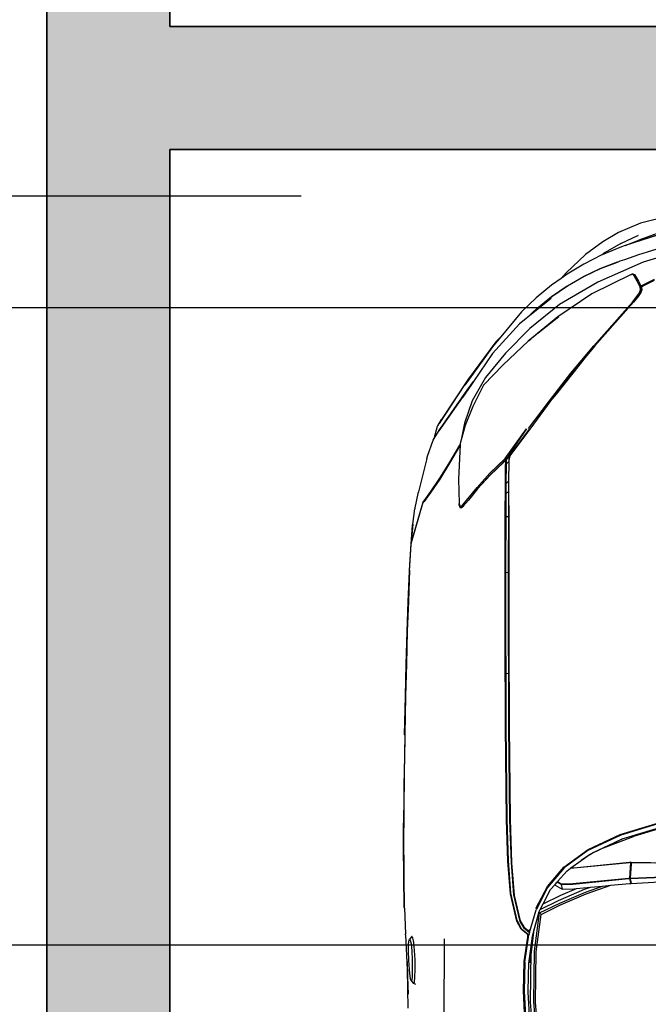
# Model space of a CAD drawing. Units: inches. Extents: x -4737294 to -4736756, y 1716389 to 1717040.
# Tile 12 of 25: x -4737217 to -4737171, y 1716597 to 1716669. Entities that reach past the tile are written whole.
import ezdxf

# ---------------------------------------------------------------- set-up
doc = ezdxf.new("R2010")
doc.units = ezdxf.units.IN
doc.header["$MEASUREMENT"] = 0
for name, color, linetype, lineweight in [('A-ANNO-DIMS', 2, 'Continuous', 18), ('A-EQPM-VEHI', 250, 'Continuous', 13), ('A-WALL-PATT', 244, 'Continuous', 13), ('walls', 252, 'Continuous', 35)]:
    doc.layers.add(name, color=color, linetype=linetype, lineweight=lineweight)
doc.layers.add('Edges', color=250, linetype='Continuous')
doc.styles.get("Standard").update_dxf_attribs({"font": 'arial.ttf'})
doc.dimstyles.get("Standard").update_dxf_attribs({"dimtxt": 8, "dimasz": 0.18, "dimexe": 0.18, "dimexo": 0.0625, "dimgap": 0.09, "dimtad": 0, "dimtih": 1, "dimtoh": 1, "dimzin": 0, "dimdsep": 46, "dimlunit": 3, "dimtxsty": 'Standard', "dimcen": 0.09, "dimadec": 0, "dimazin": 0, "dimtfac": 1, "dimtofl": 0, "dimtmove": 0, "dimatfit": 3, "dimfxl": 1, "dimtolj": 1, "dimtzin": 0, "dimarcsym": 0})

# ---------------------------------------------------------------- blocks, each defined once
blk = doc.blocks.new('Nissan Qashqai pl')
at = {"layer": 'Edges'}
for p, q in [((8.4086, 11.6764), (8.4045, 11.4011)), ((8.4305, 11.3996), (8.419, 11.6758)), ((8.4204, 11.6758), (8.4319, 11.3996)), ((8.4394, 11.4014), (8.4238, 11.6766)), ((7.3676, 11.5172), (7.3963, 11.4215)), ((8.3573, 11.3824), (8.3296, 11.4739)), ((8.3311, 11.4733), (8.3582, 11.3836)), ((8.3648, 11.3863), (8.3377, 11.4753)), ((8.3392, 11.4758), (8.3608, 11.4048)), ((7.3193, 11.4645), (7.3309, 11.4166)), ((7.344, 11.4572), (7.3596, 11.4139)), ((7.3467, 11.4596), (7.3686, 11.3913)), ((7.3489, 11.4517), (7.3686, 11.3913)), ((7.375, 11.4442), (7.3799, 11.4278)), ((7.4255, 11.4398), (7.4367, 11.4174)), ((7.4379, 11.4179), (7.4267, 11.4401)), ((8.4041, 11.4013), (8.4048, 11.4423)), ((7.3799, 11.4278), (7.3845, 11.4136)), ((7.3963, 11.4215), (7.4302, 11.3449)), ((7.3309, 11.4166), (7.347, 11.3798)), ((7.3655, 11.3837), (7.3514, 11.4133)), ((7.3686, 11.3913), (7.3596, 11.4139)), ((7.3845, 11.4136), (7.3925, 11.3899)), ((7.4167, 11.4049), (7.417, 11.4065)), ((7.4172, 11.4047), (7.4167, 11.4049)), ((7.4169, 11.4036), (7.4167, 11.4049)), ((7.4282, 11.4113), (7.4169, 11.4044)), ((7.417, 11.4065), (7.4283, 11.4135)), ((7.4183, 11.406), (7.4172, 11.4047)), ((7.4296, 11.4129), (7.4183, 11.406)), ((7.4387, 11.4162), (7.4282, 11.4113)), ((7.4283, 11.4135), (7.4359, 11.417)), ((7.4296, 11.4129), (7.4383, 11.417)), ((7.4359, 11.417), (7.4367, 11.4174)), ((7.4383, 11.417), (7.4367, 11.4174)), ((7.4375, 11.42), (7.4384, 11.4182)), ((7.4379, 11.4179), (7.4384, 11.4182)), ((7.4389, 11.4173), (7.4379, 11.4179)), ((7.4383, 11.417), (7.4379, 11.4179)), ((7.4389, 11.4173), (7.4383, 11.417)), ((7.4384, 11.4182), (7.4387, 11.4183)), ((7.4387, 11.4183), (7.443, 11.4188)), ((7.4431, 11.4166), (7.4387, 11.4162)), ((7.4389, 11.4173), (7.44, 11.4178)), ((7.4442, 11.4183), (7.44, 11.4178)), ((7.443, 11.4188), (7.4477, 11.4172)), ((7.4479, 11.4149), (7.4431, 11.4166)), ((7.4477, 11.4172), (7.4442, 11.4183)), ((7.4477, 11.4172), (7.4541, 11.4128)), ((7.4541, 11.4108), (7.4479, 11.4149)), ((7.4541, 11.4128), (7.4638, 11.4051)), ((7.4635, 11.4034), (7.4541, 11.4108)), ((7.4638, 11.4051), (7.5371, 11.34)), ((8.3799, 11.3545), (8.3608, 11.4048)), ((7.3686, 11.3913), (7.3707, 11.3849)), ((7.3925, 11.3899), (7.3938, 11.3859)), ((7.4172, 11.4047), (7.4169, 11.4044)), ((7.4169, 11.4044), (7.4169, 11.4036)), ((7.4172, 11.4018), (7.4169, 11.4036)), ((7.4169, 11.4036), (7.4169, 11.403)), ((7.4169, 11.403), (7.4172, 11.4011)), ((7.4174, 11.4013), (7.4172, 11.4018)), ((7.4172, 11.4011), (7.4498, 11.3349)), ((7.4174, 11.4013), (7.4175, 11.4012)), ((7.5369, 11.3385), (7.4635, 11.4034)), ((8.407, 11.401), (8.4037, 11.4002)), ((8.4037, 11.4002), (8.4314, 11.3985)), ((8.4037, 11.3992), (8.4037, 11.4002)), ((8.4037, 11.3992), (8.4046, 11.3981)), ((8.4042, 11.3983), (8.4037, 11.3992)), ((8.4041, 11.4013), (8.4045, 11.4011)), ((8.4134, 11.3049), (8.4042, 11.3983)), ((8.4045, 11.4011), (8.407, 11.401)), ((8.4046, 11.3981), (8.4138, 11.3048)), ((8.407, 11.401), (8.4305, 11.3996)), ((8.4305, 11.3996), (8.4319, 11.3996)), ((8.4306, 11.3966), (8.4314, 11.3975)), ((8.4398, 11.3032), (8.4306, 11.3966)), ((8.4314, 11.3985), (8.4394, 11.4004)), ((8.4314, 11.3985), (8.4314, 11.3975)), ((8.4314, 11.3975), (8.4319, 11.3967)), ((8.4319, 11.3996), (8.436, 11.4006)), ((8.4319, 11.3967), (8.4412, 11.3033)), ((8.436, 11.4006), (8.4394, 11.4014)), ((8.4394, 11.4004), (8.436, 11.4006)), ((8.4394, 11.3984), (8.4394, 11.4004)), ((8.4425, 11.3672), (8.4394, 11.3984)), ((7.347, 11.3798), (7.3624, 11.3535)), ((7.3655, 11.3837), (7.3805, 11.3576)), ((7.3707, 11.3849), (7.3843, 11.3522)), ((7.3938, 11.3859), (7.3951, 11.3822)), ((7.3951, 11.3822), (7.3965, 11.3787)), ((7.3962, 11.3781), (7.3965, 11.3787)), ((7.4071, 11.3493), (7.3962, 11.3781)), ((7.3965, 11.3787), (7.3969, 11.3777)), ((7.3969, 11.3777), (7.4078, 11.349)), ((8.3826, 11.3291), (8.3573, 11.3824)), ((8.3582, 11.3836), (8.3844, 11.3284)), ((8.3646, 11.387), (8.3799, 11.3545)), ((8.3888, 11.3355), (8.3648, 11.3863)), ((7.3805, 11.3576), (7.3843, 11.3522)), ((8.4571, 11.3258), (8.4425, 11.3672)), ((8.4439, 11.3531), (8.4425, 11.3672)), ((7.3624, 11.3535), (7.3837, 11.3245)), ((7.3843, 11.3522), (7.3845, 11.3517)), ((7.3845, 11.3517), (7.3997, 11.3215)), ((7.4205, 11.3212), (7.4071, 11.3493)), ((7.4078, 11.349), (7.4211, 11.321)), ((7.4302, 11.3449), (7.4679, 11.2807)), ((7.5371, 11.34), (7.5568, 11.324)), ((8.3799, 11.3545), (8.3888, 11.3355)), ((8.454, 11.3245), (8.4439, 11.3531)), ((8.4459, 11.3326), (8.4439, 11.3531)), ((7.3837, 11.3245), (7.4147, 11.2918)), ((7.4498, 11.3349), (7.4884, 11.2778)), ((7.5827, 11.3001), (7.5369, 11.3385)), ((7.584, 11.3013), (7.5568, 11.324)), ((7.5568, 11.324), (7.5829, 11.303)), ((8.4122, 11.2883), (8.3826, 11.3291)), ((8.3844, 11.3284), (8.4134, 11.2888)), ((8.3901, 11.3328), (8.3888, 11.3355)), ((8.3901, 11.3328), (8.4011, 11.3173)), ((8.3904, 11.3321), (8.3901, 11.3328)), ((8.4011, 11.3173), (8.3904, 11.3321)), ((8.4493, 11.3229), (8.4459, 11.3326)), ((8.4482, 11.3095), (8.4459, 11.3326)), ((8.468, 11.2793), (8.4493, 11.3229)), ((8.4725, 11.2812), (8.454, 11.3245)), ((8.4756, 11.2826), (8.4571, 11.3258)), ((7.3997, 11.3215), (7.4166, 11.2939)), ((7.4363, 11.294), (7.4205, 11.3212)), ((7.4211, 11.321), (7.4369, 11.2938)), ((8.4135, 11.3), (8.4011, 11.3173)), ((8.4594, 11.2831), (8.4482, 11.3095)), ((8.4487, 11.305), (8.4482, 11.3095)), ((7.4147, 11.2918), (7.4239, 11.2837)), ((7.4166, 11.2939), (7.4239, 11.2837)), ((7.4542, 11.2677), (7.4363, 11.294)), ((7.4369, 11.2938), (7.4549, 11.2675)), ((7.6296, 11.2639), (7.5827, 11.3001)), ((7.5829, 11.303), (7.618, 11.275)), ((7.618, 11.275), (7.584, 11.3013)), ((8.4135, 11.3), (8.4134, 11.3049)), ((8.4139, 11.2994), (8.4135, 11.3)), ((8.4138, 11.3048), (8.4139, 11.2994)), ((8.4183, 11.2934), (8.4139, 11.2994)), ((8.4365, 11.2776), (8.4183, 11.2934)), ((8.44, 11.2834), (8.4398, 11.3032)), ((8.4412, 11.3033), (8.4415, 11.2835)), ((8.4489, 11.2852), (8.4487, 11.305)), ((7.4239, 11.2837), (7.4354, 11.2675)), ((7.4679, 11.2807), (7.5081, 11.2311)), ((7.4882, 11.2797), (7.5243, 11.2341)), ((7.4884, 11.2778), (7.5289, 11.2283)), ((7.618, 11.275), (7.6301, 11.2654)), ((8.4444, 11.2608), (8.4122, 11.2883)), ((8.4134, 11.2888), (8.4462, 11.2609)), ((8.4365, 11.2776), (8.44, 11.2834)), ((8.4375, 11.2767), (8.4365, 11.2776)), ((8.4415, 11.2835), (8.4375, 11.2767)), ((8.4412, 11.2735), (8.4375, 11.2767)), ((8.4422, 11.2737), (8.4412, 11.2735)), ((8.4499, 11.2659), (8.4412, 11.2735)), ((8.4415, 11.2835), (8.4489, 11.2852)), ((8.4422, 11.2737), (8.4489, 11.2852)), ((8.4737, 11.2534), (8.4594, 11.2831)), ((8.4831, 11.2484), (8.468, 11.2793)), ((8.4889, 11.2473), (8.4725, 11.2812)), ((8.4914, 11.25), (8.4756, 11.2826)), ((7.4354, 11.2675), (7.4565, 11.2419)), ((7.4744, 11.2427), (7.4542, 11.2677)), ((7.4549, 11.2675), (7.475, 11.2426)), ((7.4574, 11.267), (7.4885, 11.2283)), ((7.676, 11.2289), (7.6296, 11.2639)), ((7.6301, 11.2654), (7.6306, 11.2651)), ((7.6306, 11.2651), (7.6306, 11.265)), ((7.6306, 11.265), (7.6373, 11.2601)), ((7.6373, 11.2601), (7.6769, 11.2312)), ((8.4814, 11.2413), (8.4444, 11.2608)), ((8.4462, 11.2609), (8.4838, 11.2415)), ((8.4737, 11.2534), (8.4499, 11.2659)), ((7.4565, 11.2419), (7.4801, 11.2168)), ((7.4918, 11.2242), (7.4744, 11.2427)), ((7.475, 11.2426), (7.477, 11.2404)), ((7.477, 11.2404), (7.4765, 11.2411)), ((7.477, 11.2405), (7.4775, 11.2399)), ((7.4784, 11.2388), (7.477, 11.2404)), ((7.477, 11.2404), (7.4775, 11.2399)), ((7.4775, 11.2399), (7.4787, 11.2385)), ((7.4775, 11.2399), (7.4787, 11.2387)), ((8.4831, 11.2484), (8.4737, 11.2534)), ((8.4867, 11.2465), (8.4831, 11.2484)), ((8.5216, 11.2303), (8.4838, 11.2415)), ((8.528, 11.2354), (8.4867, 11.2465)), ((8.5214, 11.2374), (8.4867, 11.2465)), ((8.4889, 11.2473), (8.4914, 11.25)), ((8.5531, 11.2387), (8.4889, 11.2473)), ((8.5544, 11.2416), (8.4914, 11.25)), ((8.6386, 11.2404), (8.5544, 11.2416)), ((8.7481, 11.2473), (8.6375, 11.2376)), ((8.7491, 11.2501), (8.6386, 11.2404)), ((7.4787, 11.2387), (7.4782, 11.2392)), ((7.4795, 11.2377), (7.4787, 11.2387)), ((7.4787, 11.2387), (7.4885, 11.2283)), ((7.4885, 11.2283), (7.4918, 11.2242)), ((7.4918, 11.2242), (7.5001, 11.2139)), ((7.5081, 11.2311), (7.5492, 11.1902)), ((7.5243, 11.2341), (7.5286, 11.2296)), ((7.5289, 11.2283), (7.5687, 11.1862)), ((7.7261, 11.1898), (7.6762, 11.2256)), ((7.6762, 11.2256), (7.7233, 11.1928)), ((7.6769, 11.2312), (7.7194, 11.1992)), ((7.7232, 11.1955), (7.6771, 11.2307)), ((8.5125, 11.221), (8.5177, 11.2272)), ((8.5132, 11.2202), (8.5216, 11.2303)), ((8.5155, 11.2168), (8.5258, 11.2291)), ((8.5237, 11.2252), (8.5163, 11.2162)), ((8.5197, 11.2297), (8.5166, 11.2307)), ((8.5177, 11.2272), (8.5197, 11.2297)), ((8.5216, 11.2303), (8.5197, 11.2297)), ((8.5214, 11.2374), (8.555, 11.233)), ((8.5301, 11.2352), (8.5214, 11.2374)), ((8.5216, 11.2303), (8.5258, 11.2291)), ((8.5259, 11.2279), (8.5237, 11.2252)), ((8.5258, 11.2291), (8.5259, 11.2279)), ((8.5715, 11.2227), (8.5258, 11.2291)), ((8.5294, 11.2274), (8.5259, 11.2279)), ((8.5736, 11.2291), (8.528, 11.2354)), ((8.5706, 11.2216), (8.5294, 11.2274)), ((8.6375, 11.2376), (8.5531, 11.2387)), ((8.6387, 11.2319), (8.555, 11.233)), ((8.555, 11.233), (8.5726, 11.2307)), ((8.5941, 11.2286), (8.5736, 11.2291)), ((8.5941, 11.2289), (8.5941, 11.2286)), ((8.622, 11.228), (8.5941, 11.2286)), ((8.6203, 11.2213), (8.6721, 11.2241)), ((8.6699, 11.231), (8.622, 11.228)), ((8.6721, 11.2348), (8.6387, 11.2319)), ((7.4801, 11.2168), (7.5217, 11.1823)), ((7.5001, 11.2139), (7.5501, 11.1684)), ((8.5018, 11.2098), (8.4559, 11.1991)), ((8.5029, 11.2092), (8.4571, 11.1983)), ((8.4588, 11.2036), (8.5032, 11.2141)), ((8.4595, 11.2047), (8.5025, 11.2148)), ((8.5155, 11.2168), (8.5018, 11.2098)), ((8.5025, 11.2148), (8.5125, 11.221)), ((8.5163, 11.2162), (8.5029, 11.2092)), ((8.5032, 11.2141), (8.5132, 11.2202)), ((8.6197, 11.2201), (8.5706, 11.2216)), ((8.5715, 11.2227), (8.6203, 11.2213)), ((8.6683, 11.2226), (8.6197, 11.2201)), ((7.5492, 11.1902), (7.59, 11.1565)), ((7.7194, 11.1992), (7.7232, 11.1966)), ((7.7232, 11.1966), (7.7279, 11.1965)), ((7.7281, 11.1918), (7.7232, 11.1955)), ((7.7232, 11.1955), (7.7245, 11.1955)), ((7.7267, 11.1902), (7.7233, 11.1928)), ((7.7247, 11.1954), (7.7245, 11.1955)), ((7.7245, 11.1955), (7.7294, 11.1955)), ((7.7286, 11.1881), (7.7267, 11.1902)), ((7.7281, 11.1918), (7.7299, 11.1904)), ((7.7349, 11.1917), (7.7281, 11.1918)), ((7.753, 11.1648), (7.7281, 11.1918)), ((7.7294, 11.1955), (7.731, 11.1955)), ((7.7299, 11.1904), (7.7324, 11.1876)), ((7.7299, 11.1904), (7.7364, 11.1904)), ((7.731, 11.1955), (7.7349, 11.1917)), ((7.731, 11.1955), (7.764, 11.1953)), ((7.768, 11.1915), (7.7349, 11.1917)), ((7.7363, 11.1904), (7.7364, 11.1904)), ((7.7694, 11.1901), (7.7364, 11.1904)), ((7.764, 11.1953), (7.7636, 11.1957)), ((7.768, 11.1915), (7.764, 11.1953)), ((7.764, 11.1953), (7.7662, 11.1953)), ((7.7659, 11.1957), (7.7662, 11.1953)), ((7.7662, 11.1953), (7.7668, 11.1946)), ((7.7662, 11.1953), (7.7811, 11.1952)), ((7.7692, 11.1915), (7.768, 11.1915)), ((7.7694, 11.1901), (7.7687, 11.1908)), ((7.7844, 11.1913), (7.7692, 11.1915)), ((7.7707, 11.1901), (7.7694, 11.1901)), ((7.7851, 11.19), (7.7707, 11.1901)), ((7.7811, 11.1952), (7.7809, 11.1958)), ((7.7814, 11.1946), (7.7811, 11.1952)), ((7.7811, 11.1952), (7.7822, 11.1952)), ((7.7822, 11.1952), (7.7819, 11.1958)), ((7.7822, 11.1952), (7.8057, 11.195)), ((7.7844, 11.1913), (7.7822, 11.1952)), ((7.8078, 11.1911), (7.7844, 11.1913)), ((7.7846, 11.1909), (7.7851, 11.19)), ((7.8083, 11.1898), (7.7851, 11.19)), ((7.8048, 11.1959), (7.8233, 11.1958)), ((7.8057, 11.195), (7.8233, 11.195)), ((7.8233, 11.1911), (7.8078, 11.1911)), ((7.8233, 11.195), (7.8233, 11.1958)), ((7.8233, 11.1958), (7.9014, 11.1955)), ((7.8233, 11.195), (7.902, 11.1947)), ((7.8233, 11.1911), (7.8233, 11.195)), ((7.8233, 11.1899), (7.8233, 11.1911)), ((7.9036, 11.1907), (7.8233, 11.1911)), ((7.9014, 11.1955), (7.9185, 11.1955)), ((7.902, 11.1947), (7.9183, 11.1947)), ((7.9176, 11.1908), (7.9036, 11.1907)), ((7.9183, 11.1947), (7.9176, 11.1908)), ((8.0275, 11.1909), (7.9176, 11.1908)), ((7.9185, 11.1955), (7.9183, 11.1947)), ((7.9183, 11.1947), (8.0275, 11.1948)), ((7.9185, 11.1955), (8.0273, 11.1957)), ((8.0273, 11.1957), (8.1753, 11.1963)), ((8.0275, 11.1948), (8.0876, 11.1951)), ((8.0873, 11.1911), (8.0275, 11.1909)), ((8.1753, 11.1903), (8.0276, 11.1896)), ((8.0876, 11.1951), (8.0873, 11.1911)), ((8.1755, 11.1915), (8.0873, 11.1911)), ((8.0876, 11.1951), (8.1754, 11.1954)), ((8.1753, 11.1963), (8.3318, 11.198)), ((8.3324, 11.192), (8.1753, 11.1903)), ((8.1754, 11.1954), (8.332, 11.1971)), ((8.3324, 11.1931), (8.1755, 11.1915)), ((8.3318, 11.198), (8.4049, 11.2004)), ((8.332, 11.1971), (8.4042, 11.1995)), ((8.4014, 11.1953), (8.3324, 11.1931)), ((8.4022, 11.1943), (8.3324, 11.192)), ((8.4559, 11.1991), (8.4014, 11.1953)), ((8.4571, 11.1983), (8.4022, 11.1943)), ((8.4042, 11.1995), (8.4588, 11.2036)), ((8.4049, 11.2004), (8.4595, 11.2047)), ((7.5304, 11.1737), (7.5217, 11.1823)), ((7.5217, 11.1823), (7.5387, 11.1682)), ((7.5304, 11.1737), (7.5946, 11.1262)), ((7.5687, 11.1862), (7.6032, 11.1533)), ((7.7261, 11.1898), (7.7507, 11.1638)), ((7.7507, 11.1638), (7.7286, 11.1881)), ((7.7324, 11.1876), (7.7539, 11.1642)), ((7.904, 11.1894), (7.8083, 11.1898)), ((8.0276, 11.1896), (7.904, 11.1894)), ((7.5387, 11.1682), (7.6031, 11.1217)), ((7.5501, 11.1684), (7.5969, 11.1365)), ((7.7748, 11.1423), (7.7507, 11.1638)), ((7.753, 11.1648), (7.7772, 11.1431)), ((7.7539, 11.1642), (7.7772, 11.1431)), ((7.59, 11.1565), (7.6295, 11.1344)), ((7.6032, 11.1533), (7.6386, 11.1353)), ((7.7938, 11.1271), (7.7748, 11.1423)), ((7.7772, 11.1431), (7.7959, 11.1281)), ((7.5946, 11.1262), (7.6608, 11.0825)), ((7.6113, 11.1256), (7.5969, 11.1365)), ((7.5969, 11.1365), (7.6021, 11.1329)), ((7.6021, 11.1329), (7.6118, 11.1255)), ((7.6021, 11.1329), (7.6237, 11.1181)), ((7.6759, 11.0809), (7.6113, 11.1256)), ((7.6118, 11.1255), (7.6799, 11.0783)), ((7.6295, 11.1344), (7.667, 11.1212)), ((7.6386, 11.1353), (7.6708, 11.1225)), ((7.8045, 11.1179), (7.7938, 11.1271)), ((7.7959, 11.1281), (7.8062, 11.1192)), ((7.6676, 11.0791), (7.6024, 11.1221)), ((7.667, 11.1212), (7.6949, 11.1158)), ((7.6708, 11.1225), (7.6949, 11.1158)), ((7.6949, 11.1158), (7.701, 11.1141)), ((7.701, 11.1141), (7.7024, 11.1141)), ((7.7038, 11.1132), (7.7024, 11.1141)), ((7.7024, 11.1141), (7.7034, 11.114)), ((7.7034, 11.114), (7.7056, 11.1128)), ((7.7034, 11.114), (7.7608, 11.1112)), ((7.7325, 11.0966), (7.7038, 11.1132)), ((7.7056, 11.1128), (7.7341, 11.0963)), ((7.7608, 11.1112), (7.8014, 11.1124)), ((7.8014, 11.1124), (7.8022, 11.1126)), ((7.8022, 11.1126), (7.8072, 11.1141)), ((7.8037, 11.1126), (7.8022, 11.1126)), ((7.8096, 11.1148), (7.8037, 11.1126)), ((7.8072, 11.1141), (7.8045, 11.1179)), ((7.8087, 11.1159), (7.8062, 11.1192)), ((7.8062, 11.1192), (7.8066, 11.1188)), ((7.8066, 11.1188), (7.8096, 11.1148)), ((7.8072, 11.1141), (7.8087, 11.1159)), ((7.7591, 11.08), (7.7325, 11.0966)), ((7.7341, 11.0963), (7.7606, 11.0798)), ((7.6712, 11.0767), (7.6608, 11.0825)), ((7.6721, 11.0762), (7.6712, 11.0767)), ((7.6926, 11.0705), (7.6721, 11.0762)), ((7.6793, 11.0784), (7.6759, 11.0809)), ((7.6802, 11.0782), (7.6793, 11.0784)), ((7.6802, 11.0782), (7.6799, 11.0783)), ((7.6809, 11.0777), (7.6802, 11.0782)), ((7.6926, 11.0705), (7.6809, 11.0777)), ((7.7814, 11.065), (7.7591, 11.08)), ((7.7606, 11.0798), (7.7828, 11.0649)), ((8.5326, 11.0874), (8.6675, 11.0866)), ((7.6953, 11.0688), (7.6926, 11.0705)), ((7.7223, 11.059), (7.6953, 11.0688)), ((7.7262, 11.0581), (7.7223, 11.059)), ((7.7262, 11.0581), (7.7819, 11.0438)), ((7.797, 11.0534), (7.7814, 11.065)), ((7.7828, 11.0649), (7.7984, 11.0533)), ((7.7819, 11.0438), (7.7848, 11.043)), ((7.7848, 11.043), (7.8087, 11.038)), ((7.797, 11.0534), (7.797, 11.0534)), ((7.7998, 11.0513), (7.797, 11.0534)), ((7.7984, 11.0533), (7.8007, 11.0516)), ((7.7998, 11.0513), (7.8676, 11.0318)), ((7.8007, 11.0516), (7.8002, 11.0517)), ((7.8007, 11.0516), (7.8012, 11.0513)), ((7.8681, 11.032), (7.8012, 11.0513)), ((7.8087, 11.038), (7.8106, 11.0377)), ((7.8107, 11.0377), (7.8106, 11.0377)), ((7.8363, 11.0344), (7.8107, 11.0377)), ((7.8381, 11.0342), (7.8363, 11.0344)), ((7.8363, 11.0344), (7.8676, 11.0318)), ((7.87, 11.0315), (7.8381, 11.0342)), ((7.8681, 11.032), (7.8676, 11.0318)), ((7.8681, 11.032), (7.869, 11.0317)), ((7.9137, 11.0292), (7.869, 11.0317)), ((7.9151, 11.029), (7.87, 11.0315)), ((7.9137, 11.0292), (7.9658, 11.027)), ((7.9668, 11.0268), (7.9151, 11.029)), ((7.9658, 11.027), (8.016, 11.0253)), ((8.0168, 11.0251), (7.9668, 11.0268)), ((8.016, 11.0253), (8.0713, 11.0237)), ((8.0718, 11.0235), (8.0168, 11.0251)), ((8.5259, 11.0221), (8.5838, 11.0251)), ((8.5283, 11.0336), (8.5287, 11.0329)), ((8.531, 11.0346), (8.5287, 11.0329)), ((8.5287, 11.0329), (8.5331, 11.0292)), ((8.5385, 11.0363), (8.531, 11.0346)), ((8.5331, 11.0292), (8.5346, 11.0303)), ((8.5347, 11.0282), (8.5331, 11.0292)), ((8.5346, 11.0303), (8.5406, 11.0316)), ((8.5407, 11.0274), (8.5347, 11.0282)), ((8.5518, 11.0375), (8.5385, 11.0363)), ((8.5406, 11.0316), (8.5526, 11.0328)), ((8.5527, 11.0273), (8.5407, 11.0274)), ((8.568, 11.0382), (8.5518, 11.0375)), ((8.5526, 11.0328), (8.5681, 11.0335)), ((8.5682, 11.0278), (8.5527, 11.0273)), ((8.5842, 11.0384), (8.568, 11.0382)), ((8.5681, 11.0335), (8.5836, 11.0337)), ((8.5837, 11.0288), (8.5682, 11.0278)), ((8.5707, 11.0248), (8.5965, 11.0258)), ((8.5836, 11.0337), (8.5957, 11.0334)), ((8.5958, 11.0301), (8.5837, 11.0288)), ((8.5838, 11.0251), (8.6489, 11.0263)), ((8.5838, 11.0251), (8.5965, 11.0258)), ((8.5974, 11.0381), (8.5842, 11.0384)), ((8.5957, 11.0334), (8.6017, 11.0328)), ((8.6018, 11.0312), (8.5958, 11.0301)), ((8.5965, 11.0258), (8.6252, 11.0268)), ((8.6049, 11.0373), (8.5974, 11.0381)), ((8.6017, 11.0328), (8.6032, 11.0321)), ((8.6032, 11.0321), (8.6018, 11.0312)), ((8.6073, 11.0362), (8.6032, 11.0321)), ((8.6073, 11.0362), (8.6049, 11.0373)), ((8.609, 11.0397), (8.6073, 11.0362)), ((8.0713, 11.0237), (8.1249, 11.0223)), ((8.1251, 11.0222), (8.0718, 11.0235)), ((8.1249, 11.0223), (8.1901, 11.021)), ((8.1902, 11.0208), (8.1251, 11.0222)), ((8.1901, 11.021), (8.1938, 11.021)), ((8.1902, 11.021), (8.1938, 11.021)), ((8.1904, 11.0209), (8.1902, 11.0208)), ((8.1904, 11.0209), (8.2543, 11.0198)), ((8.1938, 11.021), (8.1954, 11.0209)), ((8.1954, 11.0209), (8.2544, 11.02)), ((8.2544, 11.0198), (8.2543, 11.0199)), ((8.2543, 11.0198), (8.2544, 11.0198)), ((8.2544, 11.02), (8.3166, 11.0193)), ((8.2544, 11.0198), (8.2556, 11.0198)), ((8.2556, 11.0198), (8.256, 11.0198)), ((8.256, 11.0198), (8.2561, 11.0198)), ((8.2561, 11.0198), (8.2693, 11.0197)), ((8.2693, 11.0197), (8.2694, 11.0197)), ((8.2694, 11.0197), (8.3098, 11.0192)), ((8.3098, 11.0192), (8.3163, 11.0192)), ((8.3663, 11.019), (8.3163, 11.0192)), ((8.3597, 11.019), (8.3163, 11.0192)), ((8.3166, 11.0193), (8.3764, 11.0191)), ((8.3602, 11.019), (8.3597, 11.019)), ((8.3608, 11.019), (8.3602, 11.019)), ((8.3663, 11.019), (8.3608, 11.019)), ((8.3663, 11.019), (8.3764, 11.0191)), ((8.3757, 11.019), (8.3663, 11.019)), ((8.4282, 11.0193), (8.3757, 11.019)), ((8.3764, 11.0191), (8.4069, 11.0192)), ((8.4069, 11.0192), (8.4219, 11.0196)), ((8.4069, 11.0192), (8.4292, 11.0193)), ((8.4799, 11.0202), (8.4282, 11.0193)), ((8.4292, 11.0193), (8.4799, 11.0202)), ((8.4811, 11.0203), (8.4799, 11.0202)), ((8.4811, 11.0203), (8.5241, 11.022)), ((8.5259, 11.0221), (8.5241, 11.022))]:
    blk.add_line(p, q, dxfattribs=at)
blk = doc.blocks.new('car')
blk.add_blockref('Nissan Qashqai pl', (-9.7433, -11.9151))
blk = doc.blocks.new('*D59')
at = {"layer": 'A-ANNO-DIMS', "color": 0, "lineweight": -2, "transparency": 16777216}
for p, q in [((-4737196.539, 1716655.661), (-4737225.279, 1716655.661)), ((-4737225.099, 1716655.481), (-4737225.099, 1716564.479)), ((-4737225.099, 1716465.024), (-4737225.099, 1716556.026)), ((-4737196.539, 1716464.844), (-4737225.279, 1716464.844))]:
    blk.add_line(p, q, dxfattribs=at)
at = {"layer": 'A-ANNO-DIMS', "color": 0, "transparency": 16777216}
for points in [[(-4737225.129, 1716655.481), (-4737225.069, 1716655.481), (-4737225.099, 1716655.661)], [(-4737225.129, 1716465.024), (-4737225.069, 1716465.024), (-4737225.099, 1716464.844)]]:
    blk.add_solid(points, dxfattribs=at)
at = {"layer": 'Defpoints', "color": 0, "transparency": 16777216}
for p in [(-4737196.476, 1716655.661), (-4737225.099, 1716464.844), (-4737196.476, 1716464.844)]:
    blk.add_point(p, dxfattribs=at)
at = {"layer": 'A-ANNO-DIMS', "color": 0, "transparency": 16777216, "insert": (-4737225.099, 1716560.253), "char_height": 8, "attachment_point": 5}
blk.add_mtext('\\A1;CAR 15\'-11"', dxfattribs=at)
blk = doc.blocks.new('*D63')
at = {"layer": 'A-ANNO-DIMS', "color": 0, "lineweight": -2, "transparency": 16777216}
for p, q in [((-4737062.207, 1716647.493), (-4737270.324, 1716647.493)), ((-4737270.144, 1716647.313), (-4737270.144, 1716628.418)), ((-4737270.144, 1716601.064), (-4737270.144, 1716619.959)), ((-4737062.207, 1716600.884), (-4737270.324, 1716600.884))]:
    blk.add_line(p, q, dxfattribs=at)
at = {"layer": 'A-ANNO-DIMS', "color": 0, "transparency": 16777216}
for points in [[(-4737270.174, 1716647.313), (-4737270.114, 1716647.313), (-4737270.144, 1716647.493)], [(-4737270.174, 1716601.064), (-4737270.114, 1716601.064), (-4737270.144, 1716600.884)]]:
    blk.add_solid(points, dxfattribs=at)
at = {"layer": 'Defpoints', "color": 0, "transparency": 16777216}
for p in [(-4737270.144, 1716647.493), (-4737062.144, 1716647.493), (-4737062.144, 1716600.884)]:
    blk.add_point(p, dxfattribs=at)
at = {"layer": 'A-ANNO-DIMS', "color": 0, "transparency": 16777216, "insert": (-4737270.144, 1716624.188), "char_height": 8, "attachment_point": 5}
blk.add_mtext('\\A1;3\'-10 1/2"', dxfattribs=at)

msp = doc.modelspace()

# ---------------------------------------------------------------- hatches: boundary and pattern name
at = {"layer": 'A-WALL-PATT'}
h = msp.add_hatch(color=256, dxfattribs=at)
h.dxf.hatch_style = 1
h.paths.add_polyline_path([(-4737206.144, 1716844.565), (-4737110.144, 1716844.565), (-4737110.144, 1716823.907), (-4737105.644, 1716823.907), (-4737105.644, 1716844.565), (-4737098.44, 1716844.565), (-4737098.44, 1716849.065), (-4737206.144, 1716849.065), (-4737206.144, 1716993.065), (-4736864.144, 1716993.065), (-4736864.144, 1716849.065), (-4736963.275, 1716849.065), (-4736994.446, 1716849.065), (-4736997.144, 1716849.065), (-4736997.144, 1716844.565), (-4736864.144, 1716844.565), (-4736864.144, 1716668.565), (-4736934.391, 1716668.565), (-4736934.391, 1716664.065), (-4736864.144, 1716664.065), (-4736864.144, 1716462.065), (-4736855.144, 1716462.065), (-4736855.144, 1717002.065), (-4737215.144, 1717002.065), (-4737215.144, 1716462.065), (-4737206.144, 1716462.065), (-4737206.144, 1716659.065), (-4737062.144, 1716659.065), (-4737062.144, 1716647.493), (-4737057.644, 1716647.493), (-4737057.644, 1716796.565), (-4737071.812, 1716796.565), (-4737071.812, 1716792.065), (-4737070.805, 1716792.065), (-4737062.144, 1716792.065), (-4737062.144, 1716668.065), (-4737206.144, 1716668.065), (-4737206.144, 1716792.065), (-4737093.784, 1716792.065), (-4737093.784, 1716796.565), (-4737206.144, 1716796.565)])

# ---------------------------------------------------------------- linework, layer by layer
at = {"layer": 'walls'}
for p, q in [((-4737215.144, 1716462.065), (-4737215.144, 1717002.065)), ((-4737206.144, 1716668.065), (-4737206.144, 1716792.065)), ((-4737206.144, 1716668.065), (-4737062.144, 1716668.065)), ((-4737206.144, 1716659.065), (-4737062.144, 1716659.065)), ((-4737206.144, 1716462.065), (-4737206.144, 1716659.065))]:
    msp.add_line(p, q, dxfattribs=at)

# ---------------------------------------------------------------- block references
at = {"layer": 'A-EQPM-VEHI', "xscale": 43.56002006885659, "yscale": 43.56002006885659, "zscale": 43.56002006885659, "rotation": 270}
msp.add_blockref('car', (-4737150.017, 1716548.61), dxfattribs=at)

# ---------------------------------------------------------------- dimensions: what is measured, and where the dimension line sits
at = {"layer": 'A-ANNO-DIMS'}
dim = msp.add_linear_dim(base=(-4737225.099, 1716464.844), p1=(-4737196.476, 1716655.661), p2=(-4737196.476, 1716464.844), angle=270, text='CAR <>', dimstyle='Standard', override={"dimdec": 1, "dimlfac": 1, "dimrnd": 0, "dimzin": 1, "dimdsep": 46, "dimlunit": 4, "dimfrac": 2}, dxfattribs=at)
dim.commit()
dim.dimension.update_dxf_attribs({"geometry": '*D59', "text_midpoint": (-4737225.099, 1716560.253)})
dim = msp.add_linear_dim(base=(-4737270.144, 1716647.493), p1=(-4737062.144, 1716600.884), p2=(-4737062.144, 1716647.493), angle=90, dimstyle='Standard', override={"dimdec": 1, "dimlfac": 1, "dimrnd": 0, "dimzin": 1, "dimdsep": 46, "dimlunit": 4, "dimfrac": 2}, dxfattribs=at)
dim.commit()
dim.dimension.update_dxf_attribs({"geometry": '*D63', "text_midpoint": (-4737270.144, 1716624.188)})

doc.saveas('drawing.dxf')
